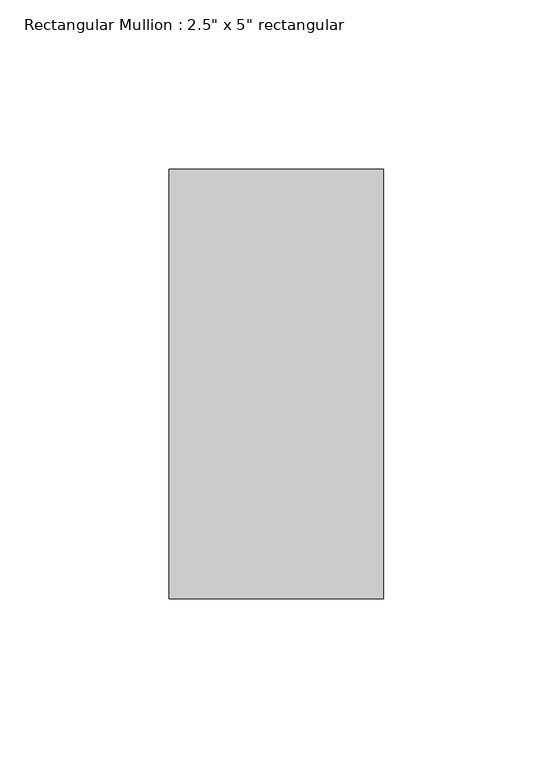
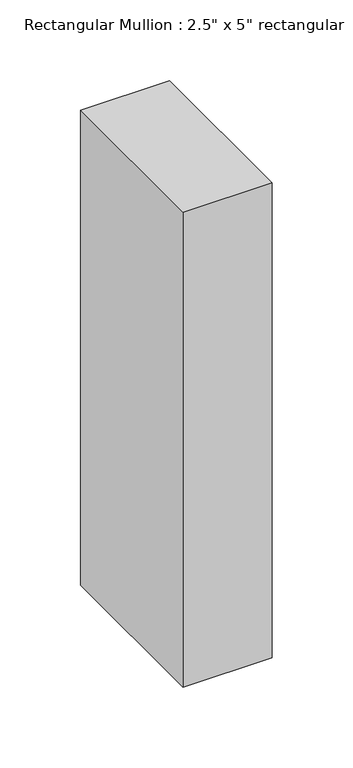
"""IFC4 building model written with IfcOpenShell, lengths in millimetres: member geometry."""

from ifc_helpers import new_model, si_unit, frame, origin, place, context, project, spatial, polyline, outline, extrude, source, transform, mapped, element, save


def member_06776a95(model_context):
    return source(origin(), model_context, "Body", "SweptSolid", [
        extrude(outline(polyline([(0.0, 63.5), (0.0, -63.5), (-63.5, -63.5), (-63.5, 63.5), (0.0, 63.5)])), frame((0.0, 0.0, -358.775), z_axis=(0.0, 0.0, 1.0), x_axis=(1.0, 0.0, 0.0)), (0.0, 0.0, 1.0), 358.775),
    ])


if __name__ == "__main__":
    model = new_model("IFC4")
    model_context = context("Model", 3, world=origin())
    ifc_project = project(units=[si_unit("LENGTHUNIT", "METRE", prefix="MILLI")], contexts=[model_context])
    site = spatial("IfcSite", under=ifc_project)
    building = spatial("IfcBuilding", under=site)
    placement = place(None, origin())
    member_shape = member_06776a95(model_context)
    element("IfcMember", 1, ObjectType="Rectangular Mullion : 2.5\" x 5\" rectangular", at=placement, inside=building, context=model_context, shape_type="MappedRepresentation", body=[
        mapped(member_shape, transform((0.0, 0.0, 0.0), x_axis=(1.0, 0.0, 0.0), y_axis=(0.0, 1.0, 0.0), z_axis=(0.0, 0.0, 1.0))),
    ])
    save(model, "model.ifc")

# Revit data of these elements
# Type "Rectangular Mullion : 2.5\" x 5\" rectangular"
#   built-in parameter 1007304 = 0.416667 (stored number, unit not read)
#   built-in parameter 1007301 = 0.104167 (stored number, unit not read)
#   built-in parameter 1007300 = 0.104167 (stored number, unit not read)
# Element 1 (IfcMember, "Rectangular Mullion : 2.5\" x 5\" rectangular")
#   Materials on its faces: "Aluminum"
# Materials
#   "Aluminum": class "Metal", colour RGB 247 247 247, transparency 0, Description = "Aluminum 6061", Cost = 0
